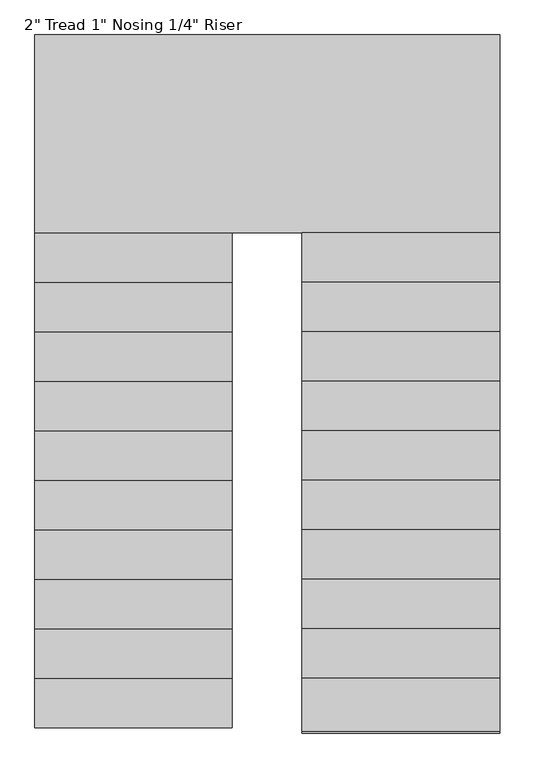
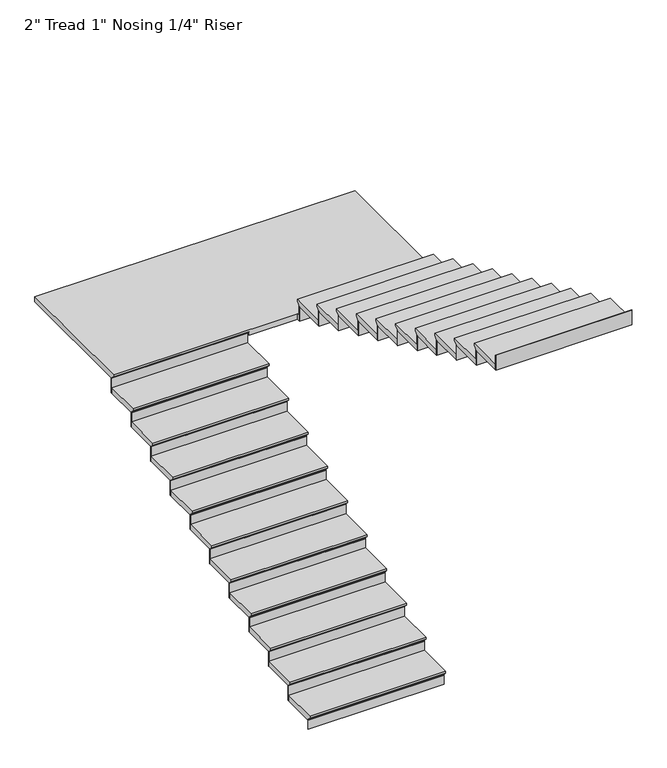
"""IFC4 building model written with IfcOpenShell, lengths in millimetres: stair flight geometry."""

from ifc_helpers import new_model, si_unit, origin, place, context, project, spatial, faceted_brep, source, transform, mapped, element, save


def stair_flight_7d9339af(model_context):
    return source(origin(), model_context, "Body", "Brep", [
        faceted_brep([(-629.5987998, 3364.6067329, 19321.8954545), (-629.5987998, 3364.6067329, 19340.9454545), (-1845.5417538, 3364.6067329, 19340.9454545), (-1845.5417538, 3364.6067329, 19321.8954545), (-629.5987998, 3390.0067329, 19296.4954545), (-1845.5417538, 3390.0067329, 19296.4954545), (-629.5987998, 3694.8067329, 19340.9454545), (-1845.5417538, 3694.8067329, 19340.9454545), (-1845.5417538, 3390.0067329, 19290.1454545), (-1845.5417538, 3694.8067329, 19290.1454545), (-629.5987998, 3694.8067329, 19290.1454545), (-629.5987998, 3390.0067329, 19290.1454545)], [[[0, 1, 2, 3]], [[4, 0, 3, 5]], [[2, 1, 6, 7]], [[8, 9, 10, 11]], [[2, 7, 9, 8, 5, 3]], [[8, 11, 4, 5]], [[6, 1, 0, 4, 11, 10]], [[7, 6, 10, 9]]]),
        faceted_brep([(-629.5987998, 3390.0067329, 19290.1454545), (-629.5987998, 3390.0067329, 19202.4), (-629.5987998, 3396.3567329, 19202.4), (-629.5987998, 3396.3567329, 19290.1454545), (-1845.5417538, 3390.0067329, 19290.1454545), (-1845.5417538, 3396.3567329, 19290.1454545), (-1845.5417538, 3396.3567329, 19202.4), (-1845.5417538, 3390.0067329, 19202.4)], [[[0, 1, 2, 3]], [[4, 5, 6, 7]], [[1, 0, 4, 7]], [[2, 1, 7, 6]], [[3, 2, 6, 5]], [[0, 3, 5, 4]]]),
        faceted_brep([(-629.5987998, 3694.8067329, 19428.6909091), (-629.5987998, 3694.8067329, 19290.1454545), (-629.5987998, 3701.1567329, 19290.1454545), (-629.5987998, 3701.1567329, 19428.6909091), (-1845.5417538, 3694.8067329, 19428.6909091), (-1845.5417538, 3701.1567329, 19428.6909091), (-1845.5417538, 3701.1567329, 19290.1454545), (-1845.5417538, 3694.8067329, 19290.1454545)], [[[0, 1, 2, 3]], [[4, 5, 6, 7]], [[1, 0, 4, 7]], [[2, 1, 7, 6]], [[3, 2, 6, 5]], [[0, 3, 5, 4]]]),
        faceted_brep([(-1845.5417538, 3669.4067329, 19479.4909091), (-629.5987998, 3669.4067329, 19479.4909091), (-629.5987998, 3999.6067329, 19479.4909091), (-1845.5417538, 3999.6067329, 19479.4909091), (-1845.5417538, 3694.8067329, 19428.6909091), (-1845.5417538, 3999.6067329, 19428.6909091), (-629.5987998, 3999.6067329, 19428.6909091), (-629.5987998, 3694.8067329, 19428.6909091), (-1845.5417538, 3694.8067329, 19435.0409091), (-1845.5417538, 3669.4067329, 19460.4409091), (-629.5987998, 3694.8067329, 19435.0409091), (-629.5987998, 3669.4067329, 19460.4409091)], [[[0, 1, 2, 3]], [[4, 5, 6, 7]], [[0, 3, 5, 4, 8, 9]], [[4, 7, 10, 8]], [[2, 1, 11, 10, 7, 6]], [[3, 2, 6, 5]], [[11, 1, 0, 9]], [[10, 11, 9, 8]]]),
        faceted_brep([(-629.5987998, 3999.6067329, 19567.2363636), (-629.5987998, 3999.6067329, 19428.6909091), (-629.5987998, 4005.9567329, 19428.6909091), (-629.5987998, 4005.9567329, 19567.2363636), (-1845.5417538, 3999.6067329, 19567.2363636), (-1845.5417538, 4005.9567329, 19567.2363636), (-1845.5417538, 4005.9567329, 19428.6909091), (-1845.5417538, 3999.6067329, 19428.6909091)], [[[0, 1, 2, 3]], [[4, 5, 6, 7]], [[1, 0, 4, 7]], [[2, 1, 7, 6]], [[3, 2, 6, 5]], [[0, 3, 5, 4]]]),
        faceted_brep([(-1845.5417538, 3974.2067329, 19618.0363636), (-629.5987998, 3974.2067329, 19618.0363636), (-629.5987998, 4304.4067329, 19618.0363636), (-1845.5417538, 4304.4067329, 19618.0363636), (-1845.5417538, 3999.6067329, 19567.2363636), (-1845.5417538, 4304.4067329, 19567.2363636), (-629.5987998, 4304.4067329, 19567.2363636), (-629.5987998, 3999.6067329, 19567.2363636), (-1845.5417538, 3999.6067329, 19573.5863636), (-1845.5417538, 3974.2067329, 19598.9863636), (-629.5987998, 3999.6067329, 19573.5863636), (-629.5987998, 3974.2067329, 19598.9863636)], [[[0, 1, 2, 3]], [[4, 5, 6, 7]], [[0, 3, 5, 4, 8, 9]], [[4, 7, 10, 8]], [[2, 1, 11, 10, 7, 6]], [[3, 2, 6, 5]], [[11, 1, 0, 9]], [[10, 11, 9, 8]]]),
        faceted_brep([(-629.5987998, 4304.4067329, 19705.7818182), (-629.5987998, 4304.4067329, 19567.2363636), (-629.5987998, 4310.7567329, 19567.2363636), (-629.5987998, 4310.7567329, 19705.7818182), (-1845.5417538, 4304.4067329, 19705.7818182), (-1845.5417538, 4310.7567329, 19705.7818182), (-1845.5417538, 4310.7567329, 19567.2363636), (-1845.5417538, 4304.4067329, 19567.2363636)], [[[0, 1, 2, 3]], [[4, 5, 6, 7]], [[1, 0, 4, 7]], [[2, 1, 7, 6]], [[3, 2, 6, 5]], [[0, 3, 5, 4]]]),
        faceted_brep([(-1845.5417538, 4279.0067329, 19756.5818182), (-629.5987998, 4279.0067329, 19756.5818182), (-629.5987998, 4609.2067329, 19756.5818182), (-1845.5417538, 4609.2067329, 19756.5818182), (-1845.5417538, 4304.4067329, 19705.7818182), (-1845.5417538, 4609.2067329, 19705.7818182), (-629.5987998, 4609.2067329, 19705.7818182), (-629.5987998, 4304.4067329, 19705.7818182), (-1845.5417538, 4304.4067329, 19712.1318182), (-1845.5417538, 4279.0067329, 19737.5318182), (-629.5987998, 4304.4067329, 19712.1318182), (-629.5987998, 4279.0067329, 19737.5318182)], [[[0, 1, 2, 3]], [[4, 5, 6, 7]], [[0, 3, 5, 4, 8, 9]], [[4, 7, 10, 8]], [[2, 1, 11, 10, 7, 6]], [[3, 2, 6, 5]], [[11, 1, 0, 9]], [[10, 11, 9, 8]]]),
        faceted_brep([(-629.5987998, 4609.2067329, 19844.3272727), (-629.5987998, 4609.2067329, 19705.7818182), (-629.5987998, 4615.5567329, 19705.7818182), (-629.5987998, 4615.5567329, 19844.3272727), (-1845.5417538, 4609.2067329, 19844.3272727), (-1845.5417538, 4615.5567329, 19844.3272727), (-1845.5417538, 4615.5567329, 19705.7818182), (-1845.5417538, 4609.2067329, 19705.7818182)], [[[0, 1, 2, 3]], [[4, 5, 6, 7]], [[1, 0, 4, 7]], [[2, 1, 7, 6]], [[3, 2, 6, 5]], [[0, 3, 5, 4]]]),
        faceted_brep([(-1845.5417538, 4583.8067329, 19895.1272727), (-629.5987998, 4583.8067329, 19895.1272727), (-629.5987998, 4914.0067329, 19895.1272727), (-1845.5417538, 4914.0067329, 19895.1272727), (-1845.5417538, 4609.2067329, 19844.3272727), (-1845.5417538, 4914.0067329, 19844.3272727), (-629.5987998, 4914.0067329, 19844.3272727), (-629.5987998, 4609.2067329, 19844.3272727), (-1845.5417538, 4609.2067329, 19850.6772727), (-1845.5417538, 4583.8067329, 19876.0772727), (-629.5987998, 4609.2067329, 19850.6772727), (-629.5987998, 4583.8067329, 19876.0772727)], [[[0, 1, 2, 3]], [[4, 5, 6, 7]], [[0, 3, 5, 4, 8, 9]], [[4, 7, 10, 8]], [[2, 1, 11, 10, 7, 6]], [[3, 2, 6, 5]], [[11, 1, 0, 9]], [[10, 11, 9, 8]]]),
        faceted_brep([(-629.5987998, 4914.0067329, 19982.8727273), (-629.5987998, 4914.0067329, 19844.3272727), (-629.5987998, 4920.3567329, 19844.3272727), (-629.5987998, 4920.3567329, 19982.8727273), (-1845.5417538, 4914.0067329, 19982.8727273), (-1845.5417538, 4920.3567329, 19982.8727273), (-1845.5417538, 4920.3567329, 19844.3272727), (-1845.5417538, 4914.0067329, 19844.3272727)], [[[0, 1, 2, 3]], [[4, 5, 6, 7]], [[1, 0, 4, 7]], [[2, 1, 7, 6]], [[3, 2, 6, 5]], [[0, 3, 5, 4]]]),
        faceted_brep([(-1845.5417538, 4888.6067329, 20033.6727273), (-629.5987998, 4888.6067329, 20033.6727273), (-629.5987998, 5218.8067329, 20033.6727273), (-1845.5417538, 5218.8067329, 20033.6727273), (-1845.5417538, 4914.0067329, 19982.8727273), (-1845.5417538, 5218.8067329, 19982.8727273), (-629.5987998, 5218.8067329, 19982.8727273), (-629.5987998, 4914.0067329, 19982.8727273), (-1845.5417538, 4914.0067329, 19989.2227273), (-1845.5417538, 4888.6067329, 20014.6227273), (-629.5987998, 4914.0067329, 19989.2227273), (-629.5987998, 4888.6067329, 20014.6227273)], [[[0, 1, 2, 3]], [[4, 5, 6, 7]], [[0, 3, 5, 4, 8, 9]], [[4, 7, 10, 8]], [[2, 1, 11, 10, 7, 6]], [[3, 2, 6, 5]], [[11, 1, 0, 9]], [[10, 11, 9, 8]]]),
        faceted_brep([(-629.5987998, 5218.8067329, 20121.4181818), (-629.5987998, 5218.8067329, 19982.8727273), (-629.5987998, 5225.1567329, 19982.8727273), (-629.5987998, 5225.1567329, 20121.4181818), (-1845.5417538, 5218.8067329, 20121.4181818), (-1845.5417538, 5225.1567329, 20121.4181818), (-1845.5417538, 5225.1567329, 19982.8727273), (-1845.5417538, 5218.8067329, 19982.8727273)], [[[0, 1, 2, 3]], [[4, 5, 6, 7]], [[1, 0, 4, 7]], [[2, 1, 7, 6]], [[3, 2, 6, 5]], [[0, 3, 5, 4]]]),
        faceted_brep([(-1845.5417538, 5193.4067329, 20172.2181818), (-629.5987998, 5193.4067329, 20172.2181818), (-629.5987998, 5523.6067329, 20172.2181818), (-1845.5417538, 5523.6067329, 20172.2181818), (-1845.5417538, 5218.8067329, 20121.4181818), (-1845.5417538, 5523.6067329, 20121.4181818), (-629.5987998, 5523.6067329, 20121.4181818), (-629.5987998, 5218.8067329, 20121.4181818), (-1845.5417538, 5218.8067329, 20127.7681818), (-1845.5417538, 5193.4067329, 20153.1681818), (-629.5987998, 5218.8067329, 20127.7681818), (-629.5987998, 5193.4067329, 20153.1681818)], [[[0, 1, 2, 3]], [[4, 5, 6, 7]], [[0, 3, 5, 4, 8, 9]], [[4, 7, 10, 8]], [[2, 1, 11, 10, 7, 6]], [[3, 2, 6, 5]], [[11, 1, 0, 9]], [[10, 11, 9, 8]]]),
        faceted_brep([(-629.5987998, 5523.6067329, 20259.9636364), (-629.5987998, 5523.6067329, 20121.4181818), (-629.5987998, 5529.9567329, 20121.4181818), (-629.5987998, 5529.9567329, 20259.9636364), (-1845.5417538, 5523.6067329, 20259.9636364), (-1845.5417538, 5529.9567329, 20259.9636364), (-1845.5417538, 5529.9567329, 20121.4181818), (-1845.5417538, 5523.6067329, 20121.4181818)], [[[0, 1, 2, 3]], [[4, 5, 6, 7]], [[1, 0, 4, 7]], [[2, 1, 7, 6]], [[3, 2, 6, 5]], [[0, 3, 5, 4]]]),
        faceted_brep([(-1845.5417538, 5498.2067329, 20310.7636364), (-629.5987998, 5498.2067329, 20310.7636364), (-629.5987998, 5828.4067329, 20310.7636364), (-1845.5417538, 5828.4067329, 20310.7636364), (-1845.5417538, 5523.6067329, 20259.9636364), (-1845.5417538, 5828.4067329, 20259.9636364), (-629.5987998, 5828.4067329, 20259.9636364), (-629.5987998, 5523.6067329, 20259.9636364), (-1845.5417538, 5523.6067329, 20266.3136364), (-1845.5417538, 5498.2067329, 20291.7136364), (-629.5987998, 5523.6067329, 20266.3136364), (-629.5987998, 5498.2067329, 20291.7136364)], [[[0, 1, 2, 3]], [[4, 5, 6, 7]], [[0, 3, 5, 4, 8, 9]], [[4, 7, 10, 8]], [[2, 1, 11, 10, 7, 6]], [[3, 2, 6, 5]], [[11, 1, 0, 9]], [[10, 11, 9, 8]]]),
        faceted_brep([(-629.5987998, 5828.4067329, 20398.5090909), (-629.5987998, 5828.4067329, 20259.9636364), (-629.5987998, 5834.7567329, 20259.9636364), (-629.5987998, 5834.7567329, 20398.5090909), (-1845.5417538, 5828.4067329, 20398.5090909), (-1845.5417538, 5834.7567329, 20398.5090909), (-1845.5417538, 5834.7567329, 20259.9636364), (-1845.5417538, 5828.4067329, 20259.9636364)], [[[0, 1, 2, 3]], [[4, 5, 6, 7]], [[1, 0, 4, 7]], [[2, 1, 7, 6]], [[3, 2, 6, 5]], [[0, 3, 5, 4]]]),
        faceted_brep([(-1845.5417538, 5803.0067329, 20449.3090909), (-629.5987998, 5803.0067329, 20449.3090909), (-629.5987998, 6133.2067329, 20449.3090909), (-1845.5417538, 6133.2067329, 20449.3090909), (-1845.5417538, 5828.4067329, 20398.5090909), (-1845.5417538, 6133.2067329, 20398.5090909), (-629.5987998, 6133.2067329, 20398.5090909), (-629.5987998, 5828.4067329, 20398.5090909), (-1845.5417538, 5828.4067329, 20404.8590909), (-1845.5417538, 5803.0067329, 20430.2590909), (-629.5987998, 5828.4067329, 20404.8590909), (-629.5987998, 5803.0067329, 20430.2590909)], [[[0, 1, 2, 3]], [[4, 5, 6, 7]], [[0, 3, 5, 4, 8, 9]], [[4, 7, 10, 8]], [[2, 1, 11, 10, 7, 6]], [[3, 2, 6, 5]], [[11, 1, 0, 9]], [[10, 11, 9, 8]]]),
        faceted_brep([(-629.5987998, 6133.2067329, 20537.0545455), (-629.5987998, 6133.2067329, 20398.5090909), (-629.5987998, 6139.5567329, 20398.5090909), (-629.5987998, 6139.5567329, 20537.0545455), (-1845.5417538, 6133.2067329, 20537.0545455), (-1845.5417538, 6139.5567329, 20537.0545455), (-1845.5417538, 6139.5567329, 20398.5090909), (-1845.5417538, 6133.2067329, 20398.5090909)], [[[0, 1, 2, 3]], [[4, 5, 6, 7]], [[1, 0, 4, 7]], [[2, 1, 7, 6]], [[3, 2, 6, 5]], [[0, 3, 5, 4]]]),
        faceted_brep([(-1845.5417538, 6107.8067329, 20587.8545455), (-629.5987998, 6107.8067329, 20587.8545455), (-629.5987998, 6438.0067329, 20587.8545455), (-1845.5417538, 6438.0067329, 20587.8545455), (-1845.5417538, 6133.2067329, 20537.0545455), (-1845.5417538, 6438.0067329, 20537.0545455), (-629.5987998, 6438.0067329, 20537.0545455), (-629.5987998, 6133.2067329, 20537.0545455), (-1845.5417538, 6133.2067329, 20543.4045455), (-1845.5417538, 6107.8067329, 20568.8045455), (-629.5987998, 6133.2067329, 20543.4045455), (-629.5987998, 6107.8067329, 20568.8045455)], [[[0, 1, 2, 3]], [[4, 5, 6, 7]], [[0, 3, 5, 4, 8, 9]], [[4, 7, 10, 8]], [[2, 1, 11, 10, 7, 6]], [[3, 2, 6, 5]], [[11, 1, 0, 9]], [[10, 11, 9, 8]]]),
        faceted_brep([(-629.5987998, 6438.0067329, 20675.6), (-629.5987998, 6438.0067329, 20537.0545455), (-629.5987998, 6444.3567329, 20537.0545455), (-629.5987998, 6444.3567329, 20675.6), (-1845.5417538, 6438.0067329, 20675.6), (-1845.5417538, 6444.3567329, 20675.6), (-1845.5417538, 6444.3567329, 20537.0545455), (-1845.5417538, 6438.0067329, 20537.0545455)], [[[0, 1, 2, 3]], [[4, 5, 6, 7]], [[1, 0, 4, 7]], [[2, 1, 7, 6]], [[3, 2, 6, 5]], [[0, 3, 5, 4]]]),
        faceted_brep([(1021.4012085, 6387.2067329, 20726.4), (1021.4012085, 7631.8067329, 20726.4), (-1845.5417538, 7631.8067329, 20726.4), (-1845.5417538, 6412.6067329, 20726.4), (-197.7987915, 6412.6067329, 20726.4), (-197.7987915, 6387.2067329, 20726.4), (1021.4012085, 7631.8067329, 20675.6), (1021.4012085, 6387.2067329, 20675.6), (-197.7987915, 6387.2067329, 20675.6), (-197.7987915, 6412.6067329, 20675.6), (-629.5987998, 6412.6067329, 20675.6), (-629.5987998, 6438.0067329, 20675.6), (-1845.5417538, 6438.0067329, 20675.6), (-1845.5417538, 7631.8067329, 20675.6), (-629.5987998, 6438.0067329, 20681.95), (-1845.5417538, 6438.0067329, 20681.95), (-1845.5417538, 6412.6067329, 20707.35), (-629.5987998, 6412.6067329, 20707.35)], [[[0, 1, 2, 3, 4, 5]], [[6, 7, 8, 9, 10, 11, 12, 13]], [[1, 0, 7, 6]], [[2, 1, 6, 13]], [[12, 11, 14, 15]], [[4, 3, 16, 17, 10, 9]], [[5, 4, 9, 8]], [[0, 5, 8, 7]], [[16, 15, 14, 17]], [[3, 2, 13, 12, 15, 16]], [[11, 10, 17, 14]]]),
        faceted_brep([(-197.7987915, 6387.2067329, 20814.1454545), (-197.7987915, 6387.2067329, 20675.6), (-197.7987915, 6380.8567329, 20675.6), (-197.7987915, 6380.8567329, 20814.1454545), (1021.4012085, 6387.2067329, 20814.1454545), (1021.4012085, 6380.8567329, 20814.1454545), (1021.4012085, 6380.8567329, 20675.6), (1021.4012085, 6387.2067329, 20675.6)], [[[0, 1, 2, 3]], [[4, 5, 6, 7]], [[1, 0, 4, 7]], [[2, 1, 7, 6]], [[3, 2, 6, 5]], [[0, 3, 5, 4]]]),
        faceted_brep([(1021.4012085, 6412.6067329, 20864.9454545), (-197.7987915, 6412.6067329, 20864.9454545), (-197.7987915, 6082.4067329, 20864.9454545), (1021.4012085, 6082.4067329, 20864.9454545), (1021.4012085, 6387.2067329, 20814.1454545), (1021.4012085, 6082.4067329, 20814.1454545), (-197.7987915, 6082.4067329, 20814.1454545), (-197.7987915, 6387.2067329, 20814.1454545), (1021.4012085, 6387.2067329, 20820.4954545), (1021.4012085, 6412.6067329, 20845.8954545), (-197.7987915, 6387.2067329, 20820.4954545), (-197.7987915, 6412.6067329, 20845.8954545)], [[[0, 1, 2, 3]], [[4, 5, 6, 7]], [[0, 3, 5, 4, 8, 9]], [[4, 7, 10, 8]], [[2, 1, 11, 10, 7, 6]], [[3, 2, 6, 5]], [[11, 1, 0, 9]], [[10, 11, 9, 8]]]),
        faceted_brep([(-197.7987915, 6082.4067329, 20952.6909091), (-197.7987915, 6082.4067329, 20814.1454545), (-197.7987915, 6076.0567329, 20814.1454545), (-197.7987915, 6076.0567329, 20952.6909091), (1021.4012085, 6082.4067329, 20952.6909091), (1021.4012085, 6076.0567329, 20952.6909091), (1021.4012085, 6076.0567329, 20814.1454545), (1021.4012085, 6082.4067329, 20814.1454545)], [[[0, 1, 2, 3]], [[4, 5, 6, 7]], [[1, 0, 4, 7]], [[2, 1, 7, 6]], [[3, 2, 6, 5]], [[0, 3, 5, 4]]]),
        faceted_brep([(1021.4012085, 6107.8067329, 21003.4909091), (-197.7987915, 6107.8067329, 21003.4909091), (-197.7987915, 5777.6067329, 21003.4909091), (1021.4012085, 5777.6067329, 21003.4909091), (1021.4012085, 6082.4067329, 20952.6909091), (1021.4012085, 5777.6067329, 20952.6909091), (-197.7987915, 5777.6067329, 20952.6909091), (-197.7987915, 6082.4067329, 20952.6909091), (1021.4012085, 6082.4067329, 20959.0409091), (1021.4012085, 6107.8067329, 20984.4409091), (-197.7987915, 6082.4067329, 20959.0409091), (-197.7987915, 6107.8067329, 20984.4409091)], [[[0, 1, 2, 3]], [[4, 5, 6, 7]], [[0, 3, 5, 4, 8, 9]], [[4, 7, 10, 8]], [[2, 1, 11, 10, 7, 6]], [[3, 2, 6, 5]], [[11, 1, 0, 9]], [[10, 11, 9, 8]]]),
        faceted_brep([(-197.7987915, 5777.6067329, 21091.2363636), (-197.7987915, 5777.6067329, 20952.6909091), (-197.7987915, 5771.2567329, 20952.6909091), (-197.7987915, 5771.2567329, 21091.2363636), (1021.4012085, 5777.6067329, 21091.2363636), (1021.4012085, 5771.2567329, 21091.2363636), (1021.4012085, 5771.2567329, 20952.6909091), (1021.4012085, 5777.6067329, 20952.6909091)], [[[0, 1, 2, 3]], [[4, 5, 6, 7]], [[1, 0, 4, 7]], [[2, 1, 7, 6]], [[3, 2, 6, 5]], [[0, 3, 5, 4]]]),
        faceted_brep([(1021.4012085, 5803.0067329, 21142.0363636), (-197.7987915, 5803.0067329, 21142.0363636), (-197.7987915, 5472.8067329, 21142.0363636), (1021.4012085, 5472.8067329, 21142.0363636), (1021.4012085, 5777.6067329, 21091.2363636), (1021.4012085, 5472.8067329, 21091.2363636), (-197.7987915, 5472.8067329, 21091.2363636), (-197.7987915, 5777.6067329, 21091.2363636), (1021.4012085, 5777.6067329, 21097.5863636), (1021.4012085, 5803.0067329, 21122.9863636), (-197.7987915, 5777.6067329, 21097.5863636), (-197.7987915, 5803.0067329, 21122.9863636)], [[[0, 1, 2, 3]], [[4, 5, 6, 7]], [[0, 3, 5, 4, 8, 9]], [[4, 7, 10, 8]], [[2, 1, 11, 10, 7, 6]], [[3, 2, 6, 5]], [[11, 1, 0, 9]], [[10, 11, 9, 8]]]),
        faceted_brep([(-197.7987915, 5472.8067329, 21229.7818182), (-197.7987915, 5472.8067329, 21091.2363636), (-197.7987915, 5466.4567329, 21091.2363636), (-197.7987915, 5466.4567329, 21229.7818182), (1021.4012085, 5472.8067329, 21229.7818182), (1021.4012085, 5466.4567329, 21229.7818182), (1021.4012085, 5466.4567329, 21091.2363636), (1021.4012085, 5472.8067329, 21091.2363636)], [[[0, 1, 2, 3]], [[4, 5, 6, 7]], [[1, 0, 4, 7]], [[2, 1, 7, 6]], [[3, 2, 6, 5]], [[0, 3, 5, 4]]]),
        faceted_brep([(1021.4012085, 5498.2067329, 21280.5818182), (-197.7987915, 5498.2067329, 21280.5818182), (-197.7987915, 5168.0067329, 21280.5818182), (1021.4012085, 5168.0067329, 21280.5818182), (1021.4012085, 5472.8067329, 21229.7818182), (1021.4012085, 5168.0067329, 21229.7818182), (-197.7987915, 5168.0067329, 21229.7818182), (-197.7987915, 5472.8067329, 21229.7818182), (1021.4012085, 5472.8067329, 21236.1318182), (1021.4012085, 5498.2067329, 21261.5318182), (-197.7987915, 5472.8067329, 21236.1318182), (-197.7987915, 5498.2067329, 21261.5318182)], [[[0, 1, 2, 3]], [[4, 5, 6, 7]], [[0, 3, 5, 4, 8, 9]], [[4, 7, 10, 8]], [[2, 1, 11, 10, 7, 6]], [[3, 2, 6, 5]], [[11, 1, 0, 9]], [[10, 11, 9, 8]]]),
        faceted_brep([(-197.7987915, 5168.0067329, 21368.3272727), (-197.7987915, 5168.0067329, 21229.7818182), (-197.7987915, 5161.6567329, 21229.7818182), (-197.7987915, 5161.6567329, 21368.3272727), (1021.4012085, 5168.0067329, 21368.3272727), (1021.4012085, 5161.6567329, 21368.3272727), (1021.4012085, 5161.6567329, 21229.7818182), (1021.4012085, 5168.0067329, 21229.7818182)], [[[0, 1, 2, 3]], [[4, 5, 6, 7]], [[1, 0, 4, 7]], [[2, 1, 7, 6]], [[3, 2, 6, 5]], [[0, 3, 5, 4]]]),
        faceted_brep([(1021.4012085, 5193.4067329, 21419.1272727), (-197.7987915, 5193.4067329, 21419.1272727), (-197.7987915, 4863.2067329, 21419.1272727), (1021.4012085, 4863.2067329, 21419.1272727), (1021.4012085, 5168.0067329, 21368.3272727), (1021.4012085, 4863.2067329, 21368.3272727), (-197.7987915, 4863.2067329, 21368.3272727), (-197.7987915, 5168.0067329, 21368.3272727), (1021.4012085, 5168.0067329, 21374.6772727), (1021.4012085, 5193.4067329, 21400.0772727), (-197.7987915, 5168.0067329, 21374.6772727), (-197.7987915, 5193.4067329, 21400.0772727)], [[[0, 1, 2, 3]], [[4, 5, 6, 7]], [[0, 3, 5, 4, 8, 9]], [[4, 7, 10, 8]], [[2, 1, 11, 10, 7, 6]], [[3, 2, 6, 5]], [[11, 1, 0, 9]], [[10, 11, 9, 8]]]),
        faceted_brep([(-197.7987915, 4863.2067329, 21506.8727273), (-197.7987915, 4863.2067329, 21368.3272727), (-197.7987915, 4856.8567329, 21368.3272727), (-197.7987915, 4856.8567329, 21506.8727273), (1021.4012085, 4863.2067329, 21506.8727273), (1021.4012085, 4856.8567329, 21506.8727273), (1021.4012085, 4856.8567329, 21368.3272727), (1021.4012085, 4863.2067329, 21368.3272727)], [[[0, 1, 2, 3]], [[4, 5, 6, 7]], [[1, 0, 4, 7]], [[2, 1, 7, 6]], [[3, 2, 6, 5]], [[0, 3, 5, 4]]]),
        faceted_brep([(1021.4012085, 4888.6067329, 21557.6727273), (-197.7987915, 4888.6067329, 21557.6727273), (-197.7987915, 4558.4067329, 21557.6727273), (1021.4012085, 4558.4067329, 21557.6727273), (1021.4012085, 4863.2067329, 21506.8727273), (1021.4012085, 4558.4067329, 21506.8727273), (-197.7987915, 4558.4067329, 21506.8727273), (-197.7987915, 4863.2067329, 21506.8727273), (1021.4012085, 4863.2067329, 21513.2227273), (1021.4012085, 4888.6067329, 21538.6227273), (-197.7987915, 4863.2067329, 21513.2227273), (-197.7987915, 4888.6067329, 21538.6227273)], [[[0, 1, 2, 3]], [[4, 5, 6, 7]], [[0, 3, 5, 4, 8, 9]], [[4, 7, 10, 8]], [[2, 1, 11, 10, 7, 6]], [[3, 2, 6, 5]], [[11, 1, 0, 9]], [[10, 11, 9, 8]]]),
        faceted_brep([(-197.7987915, 4558.4067329, 21645.4181818), (-197.7987915, 4558.4067329, 21506.8727273), (-197.7987915, 4552.0567329, 21506.8727273), (-197.7987915, 4552.0567329, 21645.4181818), (1021.4012085, 4558.4067329, 21645.4181818), (1021.4012085, 4552.0567329, 21645.4181818), (1021.4012085, 4552.0567329, 21506.8727273), (1021.4012085, 4558.4067329, 21506.8727273)], [[[0, 1, 2, 3]], [[4, 5, 6, 7]], [[1, 0, 4, 7]], [[2, 1, 7, 6]], [[3, 2, 6, 5]], [[0, 3, 5, 4]]]),
        faceted_brep([(1021.4012085, 4583.8067329, 21696.2181818), (-197.7987915, 4583.8067329, 21696.2181818), (-197.7987915, 4253.6067329, 21696.2181818), (1021.4012085, 4253.6067329, 21696.2181818), (1021.4012085, 4558.4067329, 21645.4181818), (1021.4012085, 4253.6067329, 21645.4181818), (-197.7987915, 4253.6067329, 21645.4181818), (-197.7987915, 4558.4067329, 21645.4181818), (1021.4012085, 4558.4067329, 21651.7681818), (1021.4012085, 4583.8067329, 21677.1681818), (-197.7987915, 4558.4067329, 21651.7681818), (-197.7987915, 4583.8067329, 21677.1681818)], [[[0, 1, 2, 3]], [[4, 5, 6, 7]], [[0, 3, 5, 4, 8, 9]], [[4, 7, 10, 8]], [[2, 1, 11, 10, 7, 6]], [[3, 2, 6, 5]], [[11, 1, 0, 9]], [[10, 11, 9, 8]]]),
        faceted_brep([(-197.7987915, 4253.6067329, 21783.9636364), (-197.7987915, 4253.6067329, 21645.4181818), (-197.7987915, 4247.2567329, 21645.4181818), (-197.7987915, 4247.2567329, 21783.9636364), (1021.4012085, 4253.6067329, 21783.9636364), (1021.4012085, 4247.2567329, 21783.9636364), (1021.4012085, 4247.2567329, 21645.4181818), (1021.4012085, 4253.6067329, 21645.4181818)], [[[0, 1, 2, 3]], [[4, 5, 6, 7]], [[1, 0, 4, 7]], [[2, 1, 7, 6]], [[3, 2, 6, 5]], [[0, 3, 5, 4]]]),
        faceted_brep([(1021.4012085, 4279.0067329, 21834.7636364), (-197.7987915, 4279.0067329, 21834.7636364), (-197.7987915, 3948.8067329, 21834.7636364), (1021.4012085, 3948.8067329, 21834.7636364), (1021.4012085, 4253.6067329, 21783.9636364), (1021.4012085, 3948.8067329, 21783.9636364), (-197.7987915, 3948.8067329, 21783.9636364), (-197.7987915, 4253.6067329, 21783.9636364), (1021.4012085, 4253.6067329, 21790.3136364), (1021.4012085, 4279.0067329, 21815.7136364), (-197.7987915, 4253.6067329, 21790.3136364), (-197.7987915, 4279.0067329, 21815.7136364)], [[[0, 1, 2, 3]], [[4, 5, 6, 7]], [[0, 3, 5, 4, 8, 9]], [[4, 7, 10, 8]], [[2, 1, 11, 10, 7, 6]], [[3, 2, 6, 5]], [[11, 1, 0, 9]], [[10, 11, 9, 8]]]),
        faceted_brep([(-197.7987915, 3948.8067329, 21922.5090909), (-197.7987915, 3948.8067329, 21783.9636364), (-197.7987915, 3942.4567329, 21783.9636364), (-197.7987915, 3942.4567329, 21922.5090909), (1021.4012085, 3948.8067329, 21922.5090909), (1021.4012085, 3942.4567329, 21922.5090909), (1021.4012085, 3942.4567329, 21783.9636364), (1021.4012085, 3948.8067329, 21783.9636364)], [[[0, 1, 2, 3]], [[4, 5, 6, 7]], [[1, 0, 4, 7]], [[2, 1, 7, 6]], [[3, 2, 6, 5]], [[0, 3, 5, 4]]]),
        faceted_brep([(1021.4012085, 3974.2067329, 21973.3090909), (-197.7987915, 3974.2067329, 21973.3090909), (-197.7987915, 3644.0067329, 21973.3090909), (1021.4012085, 3644.0067329, 21973.3090909), (1021.4012085, 3948.8067329, 21922.5090909), (1021.4012085, 3644.0067329, 21922.5090909), (-197.7987915, 3644.0067329, 21922.5090909), (-197.7987915, 3948.8067329, 21922.5090909), (1021.4012085, 3948.8067329, 21928.8590909), (1021.4012085, 3974.2067329, 21954.2590909), (-197.7987915, 3948.8067329, 21928.8590909), (-197.7987915, 3974.2067329, 21954.2590909)], [[[0, 1, 2, 3]], [[4, 5, 6, 7]], [[0, 3, 5, 4, 8, 9]], [[4, 7, 10, 8]], [[2, 1, 11, 10, 7, 6]], [[3, 2, 6, 5]], [[11, 1, 0, 9]], [[10, 11, 9, 8]]]),
        faceted_brep([(-197.7987915, 3644.0067329, 22061.0545455), (-197.7987915, 3644.0067329, 21922.5090909), (-197.7987915, 3637.6567329, 21922.5090909), (-197.7987915, 3637.6567329, 22061.0545455), (1021.4012085, 3644.0067329, 22061.0545455), (1021.4012085, 3637.6567329, 22061.0545455), (1021.4012085, 3637.6567329, 21922.5090909), (1021.4012085, 3644.0067329, 21922.5090909)], [[[0, 1, 2, 3]], [[4, 5, 6, 7]], [[1, 0, 4, 7]], [[2, 1, 7, 6]], [[3, 2, 6, 5]], [[0, 3, 5, 4]]]),
        faceted_brep([(-197.7987915, 3339.2067329, 22199.6), (-197.7987915, 3339.2067329, 22061.0545455), (-197.7987915, 3332.8567329, 22061.0545455), (-197.7987915, 3332.8567329, 22199.6), (1021.4012085, 3339.2067329, 22199.6), (1021.4012085, 3332.8567329, 22199.6), (1021.4012085, 3332.8567329, 22061.0545455), (1021.4012085, 3339.2067329, 22061.0545455)], [[[0, 1, 2, 3]], [[4, 5, 6, 7]], [[1, 0, 4, 7]], [[2, 1, 7, 6]], [[3, 2, 6, 5]], [[0, 3, 5, 4]]]),
        faceted_brep([(1021.4012085, 3669.4067329, 22111.8545455), (-197.7987915, 3669.4067329, 22111.8545455), (-197.7987915, 3339.2067329, 22111.8545455), (1021.4012085, 3339.2067329, 22111.8545455), (1021.4012085, 3644.0067329, 22061.0545455), (1021.4012085, 3339.2067329, 22061.0545455), (-197.7987915, 3339.2067329, 22061.0545455), (-197.7987915, 3644.0067329, 22061.0545455), (1021.4012085, 3644.0067329, 22067.4045455), (1021.4012085, 3669.4067329, 22092.8045455), (-197.7987915, 3644.0067329, 22067.4045455), (-197.7987915, 3669.4067329, 22092.8045455)], [[[0, 1, 2, 3]], [[4, 5, 6, 7]], [[0, 3, 5, 4, 8, 9]], [[4, 7, 10, 8]], [[2, 1, 11, 10, 7, 6]], [[3, 2, 6, 5]], [[11, 1, 0, 9]], [[10, 11, 9, 8]]]),
    ])


if __name__ == "__main__":
    model = new_model("IFC4")
    model_context = context("Model", 3, world=origin())
    ifc_project = project(units=[si_unit("LENGTHUNIT", "METRE", prefix="MILLI")], contexts=[model_context])
    site = spatial("IfcSite", under=ifc_project)
    building = spatial("IfcBuilding", under=site)
    placement = place(None, origin())
    stair_flight_shape = stair_flight_7d9339af(model_context)
    element("IfcStairFlight", 1, ObjectType="2\" Tread 1\" Nosing 1/4\" Riser", at=placement, inside=building, context=model_context, shape_type="MappedRepresentation", body=[
        mapped(stair_flight_shape, transform((0.0, 0.0, 0.0), x_axis=(1.0, 0.0, 0.0), y_axis=(0.0, 1.0, 0.0), z_axis=(0.0, 0.0, 1.0))),
    ])
    save(model, "model.ifc")
